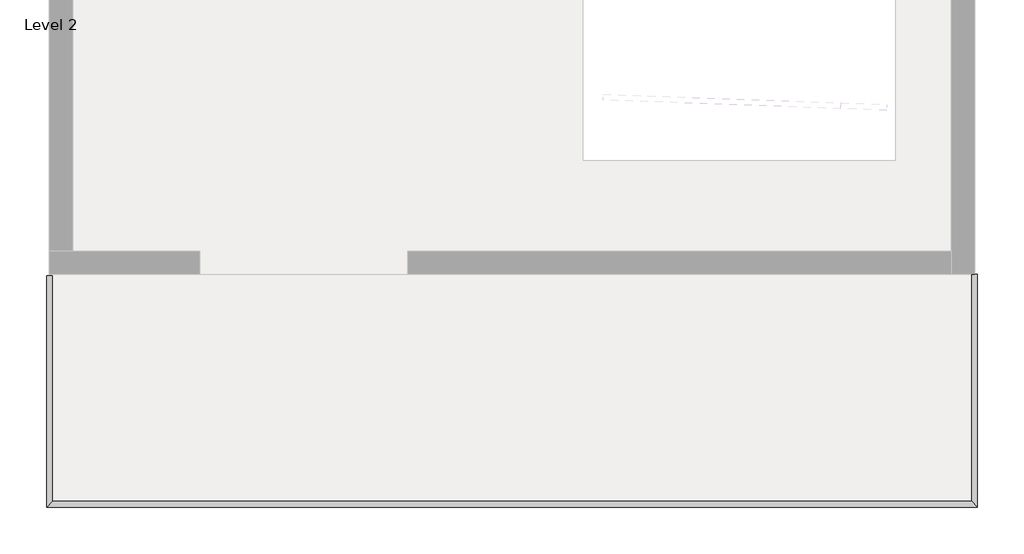
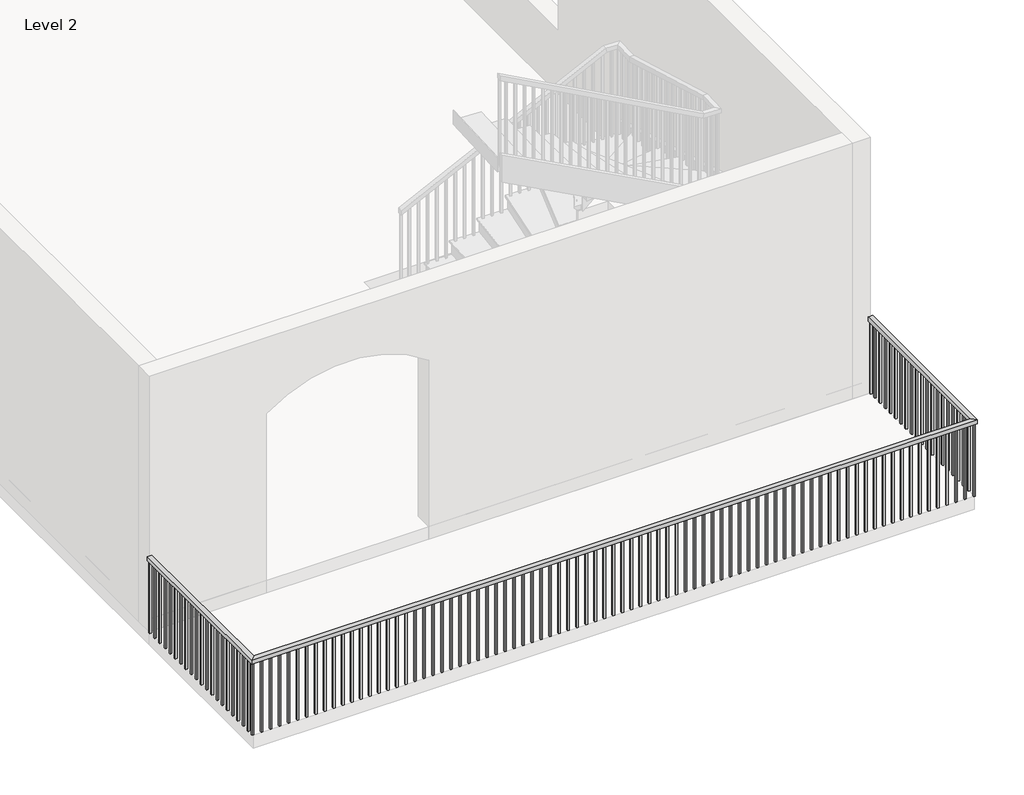
# One storey, part 2 of 3: 1 railing.
"""IFC4 building model written with IfcOpenShell, lengths in millimetres."""

from ifc_helpers import new_model, si_unit, frame, origin, place, context, project, spatial, polyline, outline, extrude, faceted_brep, element, save

model = new_model("IFC4")

# Units and contexts
model_context = context("Model", 3, world=origin())
ifc_project = project(units=[si_unit("LENGTHUNIT", "METRE", prefix="MILLI")], contexts=[model_context])

# Site, building, storey
site = spatial("IfcSite", under=ifc_project)
building = spatial("IfcBuilding", under=site)
storey = spatial("IfcBuildingStorey", under=building, Name="Level 2", Elevation=3048.0)

# Railing
placement = place(None, origin())
element("IfcRailing", 1, ObjectType="Handrail - Rectangular", at=placement, inside=storey, context=model_context, shape_type="SolidModel", body=[
    faceted_brep([(-14924.1126504, -4064.508, 3962.4), (-14924.1126504, -4064.508, 3911.6), (-14974.9126504, -4064.508, 3911.6), (-14974.9126504, -4064.508, 3962.4), (-14924.1126504, -6045.708, 3962.4), (-14924.1126504, -6045.708, 3911.6), (-14974.9126504, -6096.508, 3911.6), (-14974.9126504, -6096.508, 3962.4), (-6846.9126504, -6045.708, 3962.4), (-6846.9126504, -6045.708, 3911.6), (-6796.1126504, -6096.508, 3911.6), (-6796.1126504, -6096.508, 3962.4), (-6846.9126504, -4050.471143, 3962.4), (-6796.1126504, -4050.471143, 3962.4), (-6796.1126504, -4050.471143, 3911.6), (-6846.9126504, -4050.471143, 3911.6)], [[[0, 1, 2, 3]], [[1, 0, 4, 5]], [[2, 1, 5, 6]], [[3, 2, 6, 7]], [[0, 3, 7, 4]], [[5, 4, 8, 9]], [[6, 5, 9, 10]], [[7, 6, 10, 11]], [[4, 7, 11, 8]], [[12, 13, 14, 15]], [[9, 8, 12, 15]], [[10, 9, 15, 14]], [[11, 10, 14, 13]], [[8, 11, 13, 12]]]),
    extrude(outline(polyline([(-6811.9876504, -4150.233), (-6831.0376504, -4150.233), (-6831.0376504, -4131.183), (-6811.9876504, -4131.183), (-6811.9876504, -4150.233)])), frame((0.0, 0.0, 3048.0), z_axis=(0.0, 0.0, 1.0), x_axis=(1.0, 0.0, 0.0)), (0.0, 0.0, 1.0), 863.6),
    extrude(outline(polyline([(-6811.9876504, -4251.833), (-6831.0376504, -4251.833), (-6831.0376504, -4232.783), (-6811.9876504, -4232.783), (-6811.9876504, -4251.833)])), frame((0.0, 0.0, 3048.0), z_axis=(0.0, 0.0, 1.0), x_axis=(1.0, 0.0, 0.0)), (0.0, 0.0, 1.0), 863.6),
    extrude(outline(polyline([(-6811.9876504, -4353.433), (-6831.0376504, -4353.433), (-6831.0376504, -4334.383), (-6811.9876504, -4334.383), (-6811.9876504, -4353.433)])), frame((0.0, 0.0, 3048.0), z_axis=(0.0, 0.0, 1.0), x_axis=(1.0, 0.0, 0.0)), (0.0, 0.0, 1.0), 863.6),
    extrude(outline(polyline([(-6811.9876504, -4455.033), (-6831.0376504, -4455.033), (-6831.0376504, -4435.983), (-6811.9876504, -4435.983), (-6811.9876504, -4455.033)])), frame((0.0, 0.0, 3048.0), z_axis=(0.0, 0.0, 1.0), x_axis=(1.0, 0.0, 0.0)), (0.0, 0.0, 1.0), 863.6),
    extrude(outline(polyline([(-6811.9876504, -4556.633), (-6831.0376504, -4556.633), (-6831.0376504, -4537.583), (-6811.9876504, -4537.583), (-6811.9876504, -4556.633)])), frame((0.0, 0.0, 3048.0), z_axis=(0.0, 0.0, 1.0), x_axis=(1.0, 0.0, 0.0)), (0.0, 0.0, 1.0), 863.6),
    extrude(outline(polyline([(-6811.9876504, -4658.233), (-6831.0376504, -4658.233), (-6831.0376504, -4639.183), (-6811.9876504, -4639.183), (-6811.9876504, -4658.233)])), frame((0.0, 0.0, 3048.0), z_axis=(0.0, 0.0, 1.0), x_axis=(1.0, 0.0, 0.0)), (0.0, 0.0, 1.0), 863.6),
    extrude(outline(polyline([(-6811.9876504, -4759.833), (-6831.0376504, -4759.833), (-6831.0376504, -4740.783), (-6811.9876504, -4740.783), (-6811.9876504, -4759.833)])), frame((0.0, 0.0, 3048.0), z_axis=(0.0, 0.0, 1.0), x_axis=(1.0, 0.0, 0.0)), (0.0, 0.0, 1.0), 863.6),
    extrude(outline(polyline([(-6811.9876504, -4861.433), (-6831.0376504, -4861.433), (-6831.0376504, -4842.383), (-6811.9876504, -4842.383), (-6811.9876504, -4861.433)])), frame((0.0, 0.0, 3048.0), z_axis=(0.0, 0.0, 1.0), x_axis=(1.0, 0.0, 0.0)), (0.0, 0.0, 1.0), 863.6),
    extrude(outline(polyline([(-6811.9876504, -4963.033), (-6831.0376504, -4963.033), (-6831.0376504, -4943.983), (-6811.9876504, -4943.983), (-6811.9876504, -4963.033)])), frame((0.0, 0.0, 3048.0), z_axis=(0.0, 0.0, 1.0), x_axis=(1.0, 0.0, 0.0)), (0.0, 0.0, 1.0), 863.6),
    extrude(outline(polyline([(-6811.9876504, -5064.633), (-6831.0376504, -5064.633), (-6831.0376504, -5045.583), (-6811.9876504, -5045.583), (-6811.9876504, -5064.633)])), frame((0.0, 0.0, 3048.0), z_axis=(0.0, 0.0, 1.0), x_axis=(1.0, 0.0, 0.0)), (0.0, 0.0, 1.0), 863.6),
    extrude(outline(polyline([(-6811.9876504, -5166.233), (-6831.0376504, -5166.233), (-6831.0376504, -5147.183), (-6811.9876504, -5147.183), (-6811.9876504, -5166.233)])), frame((0.0, 0.0, 3048.0), z_axis=(0.0, 0.0, 1.0), x_axis=(1.0, 0.0, 0.0)), (0.0, 0.0, 1.0), 863.6),
    extrude(outline(polyline([(-6811.9876504, -5267.833), (-6831.0376504, -5267.833), (-6831.0376504, -5248.783), (-6811.9876504, -5248.783), (-6811.9876504, -5267.833)])), frame((0.0, 0.0, 3048.0), z_axis=(0.0, 0.0, 1.0), x_axis=(1.0, 0.0, 0.0)), (0.0, 0.0, 1.0), 863.6),
    extrude(outline(polyline([(-6811.9876504, -5369.433), (-6831.0376504, -5369.433), (-6831.0376504, -5350.383), (-6811.9876504, -5350.383), (-6811.9876504, -5369.433)])), frame((0.0, 0.0, 3048.0), z_axis=(0.0, 0.0, 1.0), x_axis=(1.0, 0.0, 0.0)), (0.0, 0.0, 1.0), 863.6),
    extrude(outline(polyline([(-6811.9876504, -5471.033), (-6831.0376504, -5471.033), (-6831.0376504, -5451.983), (-6811.9876504, -5451.983), (-6811.9876504, -5471.033)])), frame((0.0, 0.0, 3048.0), z_axis=(0.0, 0.0, 1.0), x_axis=(1.0, 0.0, 0.0)), (0.0, 0.0, 1.0), 863.6),
    extrude(outline(polyline([(-6811.9876504, -5572.633), (-6831.0376504, -5572.633), (-6831.0376504, -5553.583), (-6811.9876504, -5553.583), (-6811.9876504, -5572.633)])), frame((0.0, 0.0, 3048.0), z_axis=(0.0, 0.0, 1.0), x_axis=(1.0, 0.0, 0.0)), (0.0, 0.0, 1.0), 863.6),
    extrude(outline(polyline([(-6811.9876504, -5674.233), (-6831.0376504, -5674.233), (-6831.0376504, -5655.183), (-6811.9876504, -5655.183), (-6811.9876504, -5674.233)])), frame((0.0, 0.0, 3048.0), z_axis=(0.0, 0.0, 1.0), x_axis=(1.0, 0.0, 0.0)), (0.0, 0.0, 1.0), 863.6),
    extrude(outline(polyline([(-6811.9876504, -5775.833), (-6831.0376504, -5775.833), (-6831.0376504, -5756.783), (-6811.9876504, -5756.783), (-6811.9876504, -5775.833)])), frame((0.0, 0.0, 3048.0), z_axis=(0.0, 0.0, 1.0), x_axis=(1.0, 0.0, 0.0)), (0.0, 0.0, 1.0), 863.6),
    extrude(outline(polyline([(-6811.9876504, -5877.433), (-6831.0376504, -5877.433), (-6831.0376504, -5858.383), (-6811.9876504, -5858.383), (-6811.9876504, -5877.433)])), frame((0.0, 0.0, 3048.0), z_axis=(0.0, 0.0, 1.0), x_axis=(1.0, 0.0, 0.0)), (0.0, 0.0, 1.0), 863.6),
    extrude(outline(polyline([(-6811.9876504, -5979.033), (-6831.0376504, -5979.033), (-6831.0376504, -5959.983), (-6811.9876504, -5959.983), (-6811.9876504, -5979.033)])), frame((0.0, 0.0, 3048.0), z_axis=(0.0, 0.0, 1.0), x_axis=(1.0, 0.0, 0.0)), (0.0, 0.0, 1.0), 863.6),
    extrude(outline(polyline([(-6932.6376504, -6080.633), (-6932.6376504, -6061.583), (-6913.5876504, -6061.583), (-6913.5876504, -6080.633), (-6932.6376504, -6080.633)])), frame((0.0, 0.0, 3048.0), z_axis=(0.0, 0.0, 1.0), x_axis=(1.0, 0.0, 0.0)), (0.0, 0.0, 1.0), 863.6),
    extrude(outline(polyline([(-7034.2376504, -6080.633), (-7034.2376504, -6061.583), (-7015.1876504, -6061.583), (-7015.1876504, -6080.633), (-7034.2376504, -6080.633)])), frame((0.0, 0.0, 3048.0), z_axis=(0.0, 0.0, 1.0), x_axis=(1.0, 0.0, 0.0)), (0.0, 0.0, 1.0), 863.6),
    extrude(outline(polyline([(-7135.8376504, -6080.633), (-7135.8376504, -6061.583), (-7116.7876504, -6061.583), (-7116.7876504, -6080.633), (-7135.8376504, -6080.633)])), frame((0.0, 0.0, 3048.0), z_axis=(0.0, 0.0, 1.0), x_axis=(1.0, 0.0, 0.0)), (0.0, 0.0, 1.0), 863.6),
    extrude(outline(polyline([(-7237.4376504, -6080.633), (-7237.4376504, -6061.583), (-7218.3876504, -6061.583), (-7218.3876504, -6080.633), (-7237.4376504, -6080.633)])), frame((0.0, 0.0, 3048.0), z_axis=(0.0, 0.0, 1.0), x_axis=(1.0, 0.0, 0.0)), (0.0, 0.0, 1.0), 863.6),
    extrude(outline(polyline([(-7339.0376504, -6080.633), (-7339.0376504, -6061.583), (-7319.9876504, -6061.583), (-7319.9876504, -6080.633), (-7339.0376504, -6080.633)])), frame((0.0, 0.0, 3048.0), z_axis=(0.0, 0.0, 1.0), x_axis=(1.0, 0.0, 0.0)), (0.0, 0.0, 1.0), 863.6),
    extrude(outline(polyline([(-7440.6376504, -6080.633), (-7440.6376504, -6061.583), (-7421.5876504, -6061.583), (-7421.5876504, -6080.633), (-7440.6376504, -6080.633)])), frame((0.0, 0.0, 3048.0), z_axis=(0.0, 0.0, 1.0), x_axis=(1.0, 0.0, 0.0)), (0.0, 0.0, 1.0), 863.6),
    extrude(outline(polyline([(-7542.2376504, -6080.633), (-7542.2376504, -6061.583), (-7523.1876504, -6061.583), (-7523.1876504, -6080.633), (-7542.2376504, -6080.633)])), frame((0.0, 0.0, 3048.0), z_axis=(0.0, 0.0, 1.0), x_axis=(1.0, 0.0, 0.0)), (0.0, 0.0, 1.0), 863.6),
    extrude(outline(polyline([(-7643.8376504, -6080.633), (-7643.8376504, -6061.583), (-7624.7876504, -6061.583), (-7624.7876504, -6080.633), (-7643.8376504, -6080.633)])), frame((0.0, 0.0, 3048.0), z_axis=(0.0, 0.0, 1.0), x_axis=(1.0, 0.0, 0.0)), (0.0, 0.0, 1.0), 863.6),
    extrude(outline(polyline([(-7745.4376504, -6080.633), (-7745.4376504, -6061.583), (-7726.3876504, -6061.583), (-7726.3876504, -6080.633), (-7745.4376504, -6080.633)])), frame((0.0, 0.0, 3048.0), z_axis=(0.0, 0.0, 1.0), x_axis=(1.0, 0.0, 0.0)), (0.0, 0.0, 1.0), 863.6),
    extrude(outline(polyline([(-7847.0376504, -6080.633), (-7847.0376504, -6061.583), (-7827.9876504, -6061.583), (-7827.9876504, -6080.633), (-7847.0376504, -6080.633)])), frame((0.0, 0.0, 3048.0), z_axis=(0.0, 0.0, 1.0), x_axis=(1.0, 0.0, 0.0)), (0.0, 0.0, 1.0), 863.6),
    extrude(outline(polyline([(-7948.6376504, -6080.633), (-7948.6376504, -6061.583), (-7929.5876504, -6061.583), (-7929.5876504, -6080.633), (-7948.6376504, -6080.633)])), frame((0.0, 0.0, 3048.0), z_axis=(0.0, 0.0, 1.0), x_axis=(1.0, 0.0, 0.0)), (0.0, 0.0, 1.0), 863.6),
    extrude(outline(polyline([(-8050.2376504, -6080.633), (-8050.2376504, -6061.583), (-8031.1876504, -6061.583), (-8031.1876504, -6080.633), (-8050.2376504, -6080.633)])), frame((0.0, 0.0, 3048.0), z_axis=(0.0, 0.0, 1.0), x_axis=(1.0, 0.0, 0.0)), (0.0, 0.0, 1.0), 863.6),
    extrude(outline(polyline([(-8151.8376504, -6080.633), (-8151.8376504, -6061.583), (-8132.7876504, -6061.583), (-8132.7876504, -6080.633), (-8151.8376504, -6080.633)])), frame((0.0, 0.0, 3048.0), z_axis=(0.0, 0.0, 1.0), x_axis=(1.0, 0.0, 0.0)), (0.0, 0.0, 1.0), 863.6),
    extrude(outline(polyline([(-8253.4376504, -6080.633), (-8253.4376504, -6061.583), (-8234.3876504, -6061.583), (-8234.3876504, -6080.633), (-8253.4376504, -6080.633)])), frame((0.0, 0.0, 3048.0), z_axis=(0.0, 0.0, 1.0), x_axis=(1.0, 0.0, 0.0)), (0.0, 0.0, 1.0), 863.6),
    extrude(outline(polyline([(-8355.0376504, -6080.633), (-8355.0376504, -6061.583), (-8335.9876504, -6061.583), (-8335.9876504, -6080.633), (-8355.0376504, -6080.633)])), frame((0.0, 0.0, 3048.0), z_axis=(0.0, 0.0, 1.0), x_axis=(1.0, 0.0, 0.0)), (0.0, 0.0, 1.0), 863.6),
    extrude(outline(polyline([(-8456.6376504, -6080.633), (-8456.6376504, -6061.583), (-8437.5876504, -6061.583), (-8437.5876504, -6080.633), (-8456.6376504, -6080.633)])), frame((0.0, 0.0, 3048.0), z_axis=(0.0, 0.0, 1.0), x_axis=(1.0, 0.0, 0.0)), (0.0, 0.0, 1.0), 863.6),
    extrude(outline(polyline([(-8558.2376504, -6080.633), (-8558.2376504, -6061.583), (-8539.1876504, -6061.583), (-8539.1876504, -6080.633), (-8558.2376504, -6080.633)])), frame((0.0, 0.0, 3048.0), z_axis=(0.0, 0.0, 1.0), x_axis=(1.0, 0.0, 0.0)), (0.0, 0.0, 1.0), 863.6),
    extrude(outline(polyline([(-8659.8376504, -6080.633), (-8659.8376504, -6061.583), (-8640.7876504, -6061.583), (-8640.7876504, -6080.633), (-8659.8376504, -6080.633)])), frame((0.0, 0.0, 3048.0), z_axis=(0.0, 0.0, 1.0), x_axis=(1.0, 0.0, 0.0)), (0.0, 0.0, 1.0), 863.6),
    extrude(outline(polyline([(-8761.4376504, -6080.633), (-8761.4376504, -6061.583), (-8742.3876504, -6061.583), (-8742.3876504, -6080.633), (-8761.4376504, -6080.633)])), frame((0.0, 0.0, 3048.0), z_axis=(0.0, 0.0, 1.0), x_axis=(1.0, 0.0, 0.0)), (0.0, 0.0, 1.0), 863.6),
    extrude(outline(polyline([(-8863.0376504, -6080.633), (-8863.0376504, -6061.583), (-8843.9876504, -6061.583), (-8843.9876504, -6080.633), (-8863.0376504, -6080.633)])), frame((0.0, 0.0, 3048.0), z_axis=(0.0, 0.0, 1.0), x_axis=(1.0, 0.0, 0.0)), (0.0, 0.0, 1.0), 863.6),
    extrude(outline(polyline([(-8964.6376504, -6080.633), (-8964.6376504, -6061.583), (-8945.5876504, -6061.583), (-8945.5876504, -6080.633), (-8964.6376504, -6080.633)])), frame((0.0, 0.0, 3048.0), z_axis=(0.0, 0.0, 1.0), x_axis=(1.0, 0.0, 0.0)), (0.0, 0.0, 1.0), 863.6),
    extrude(outline(polyline([(-9066.2376504, -6080.633), (-9066.2376504, -6061.583), (-9047.1876504, -6061.583), (-9047.1876504, -6080.633), (-9066.2376504, -6080.633)])), frame((0.0, 0.0, 3048.0), z_axis=(0.0, 0.0, 1.0), x_axis=(1.0, 0.0, 0.0)), (0.0, 0.0, 1.0), 863.6),
    extrude(outline(polyline([(-9167.8376504, -6080.633), (-9167.8376504, -6061.583), (-9148.7876504, -6061.583), (-9148.7876504, -6080.633), (-9167.8376504, -6080.633)])), frame((0.0, 0.0, 3048.0), z_axis=(0.0, 0.0, 1.0), x_axis=(1.0, 0.0, 0.0)), (0.0, 0.0, 1.0), 863.6),
    extrude(outline(polyline([(-9269.4376504, -6080.633), (-9269.4376504, -6061.583), (-9250.3876504, -6061.583), (-9250.3876504, -6080.633), (-9269.4376504, -6080.633)])), frame((0.0, 0.0, 3048.0), z_axis=(0.0, 0.0, 1.0), x_axis=(1.0, 0.0, 0.0)), (0.0, 0.0, 1.0), 863.6),
    extrude(outline(polyline([(-9371.0376504, -6080.633), (-9371.0376504, -6061.583), (-9351.9876504, -6061.583), (-9351.9876504, -6080.633), (-9371.0376504, -6080.633)])), frame((0.0, 0.0, 3048.0), z_axis=(0.0, 0.0, 1.0), x_axis=(1.0, 0.0, 0.0)), (0.0, 0.0, 1.0), 863.6),
    extrude(outline(polyline([(-9472.6376504, -6080.633), (-9472.6376504, -6061.583), (-9453.5876504, -6061.583), (-9453.5876504, -6080.633), (-9472.6376504, -6080.633)])), frame((0.0, 0.0, 3048.0), z_axis=(0.0, 0.0, 1.0), x_axis=(1.0, 0.0, 0.0)), (0.0, 0.0, 1.0), 863.6),
    extrude(outline(polyline([(-9574.2376504, -6080.633), (-9574.2376504, -6061.583), (-9555.1876504, -6061.583), (-9555.1876504, -6080.633), (-9574.2376504, -6080.633)])), frame((0.0, 0.0, 3048.0), z_axis=(0.0, 0.0, 1.0), x_axis=(1.0, 0.0, 0.0)), (0.0, 0.0, 1.0), 863.6),
    extrude(outline(polyline([(-9675.8376504, -6080.633), (-9675.8376504, -6061.583), (-9656.7876504, -6061.583), (-9656.7876504, -6080.633), (-9675.8376504, -6080.633)])), frame((0.0, 0.0, 3048.0), z_axis=(0.0, 0.0, 1.0), x_axis=(1.0, 0.0, 0.0)), (0.0, 0.0, 1.0), 863.6),
    extrude(outline(polyline([(-9777.4376504, -6080.633), (-9777.4376504, -6061.583), (-9758.3876504, -6061.583), (-9758.3876504, -6080.633), (-9777.4376504, -6080.633)])), frame((0.0, 0.0, 3048.0), z_axis=(0.0, 0.0, 1.0), x_axis=(1.0, 0.0, 0.0)), (0.0, 0.0, 1.0), 863.6),
    extrude(outline(polyline([(-9879.0376504, -6080.633), (-9879.0376504, -6061.583), (-9859.9876504, -6061.583), (-9859.9876504, -6080.633), (-9879.0376504, -6080.633)])), frame((0.0, 0.0, 3048.0), z_axis=(0.0, 0.0, 1.0), x_axis=(1.0, 0.0, 0.0)), (0.0, 0.0, 1.0), 863.6),
    extrude(outline(polyline([(-9980.6376504, -6080.633), (-9980.6376504, -6061.583), (-9961.5876504, -6061.583), (-9961.5876504, -6080.633), (-9980.6376504, -6080.633)])), frame((0.0, 0.0, 3048.0), z_axis=(0.0, 0.0, 1.0), x_axis=(1.0, 0.0, 0.0)), (0.0, 0.0, 1.0), 863.6),
    extrude(outline(polyline([(-10082.2376504, -6080.633), (-10082.2376504, -6061.583), (-10063.1876504, -6061.583), (-10063.1876504, -6080.633), (-10082.2376504, -6080.633)])), frame((0.0, 0.0, 3048.0), z_axis=(0.0, 0.0, 1.0), x_axis=(1.0, 0.0, 0.0)), (0.0, 0.0, 1.0), 863.6),
    extrude(outline(polyline([(-10183.8376504, -6080.633), (-10183.8376504, -6061.583), (-10164.7876504, -6061.583), (-10164.7876504, -6080.633), (-10183.8376504, -6080.633)])), frame((0.0, 0.0, 3048.0), z_axis=(0.0, 0.0, 1.0), x_axis=(1.0, 0.0, 0.0)), (0.0, 0.0, 1.0), 863.6),
    extrude(outline(polyline([(-10285.4376504, -6080.633), (-10285.4376504, -6061.583), (-10266.3876504, -6061.583), (-10266.3876504, -6080.633), (-10285.4376504, -6080.633)])), frame((0.0, 0.0, 3048.0), z_axis=(0.0, 0.0, 1.0), x_axis=(1.0, 0.0, 0.0)), (0.0, 0.0, 1.0), 863.6),
    extrude(outline(polyline([(-10387.0376504, -6080.633), (-10387.0376504, -6061.583), (-10367.9876504, -6061.583), (-10367.9876504, -6080.633), (-10387.0376504, -6080.633)])), frame((0.0, 0.0, 3048.0), z_axis=(0.0, 0.0, 1.0), x_axis=(1.0, 0.0, 0.0)), (0.0, 0.0, 1.0), 863.6),
    extrude(outline(polyline([(-10488.6376504, -6080.633), (-10488.6376504, -6061.583), (-10469.5876504, -6061.583), (-10469.5876504, -6080.633), (-10488.6376504, -6080.633)])), frame((0.0, 0.0, 3048.0), z_axis=(0.0, 0.0, 1.0), x_axis=(1.0, 0.0, 0.0)), (0.0, 0.0, 1.0), 863.6),
    extrude(outline(polyline([(-10590.2376504, -6080.633), (-10590.2376504, -6061.583), (-10571.1876504, -6061.583), (-10571.1876504, -6080.633), (-10590.2376504, -6080.633)])), frame((0.0, 0.0, 3048.0), z_axis=(0.0, 0.0, 1.0), x_axis=(1.0, 0.0, 0.0)), (0.0, 0.0, 1.0), 863.6),
    extrude(outline(polyline([(-10691.8376504, -6080.633), (-10691.8376504, -6061.583), (-10672.7876504, -6061.583), (-10672.7876504, -6080.633), (-10691.8376504, -6080.633)])), frame((0.0, 0.0, 3048.0), z_axis=(0.0, 0.0, 1.0), x_axis=(1.0, 0.0, 0.0)), (0.0, 0.0, 1.0), 863.6),
    extrude(outline(polyline([(-10793.4376504, -6080.633), (-10793.4376504, -6061.583), (-10774.3876504, -6061.583), (-10774.3876504, -6080.633), (-10793.4376504, -6080.633)])), frame((0.0, 0.0, 3048.0), z_axis=(0.0, 0.0, 1.0), x_axis=(1.0, 0.0, 0.0)), (0.0, 0.0, 1.0), 863.6),
    extrude(outline(polyline([(-10895.0376504, -6080.633), (-10895.0376504, -6061.583), (-10875.9876504, -6061.583), (-10875.9876504, -6080.633), (-10895.0376504, -6080.633)])), frame((0.0, 0.0, 3048.0), z_axis=(0.0, 0.0, 1.0), x_axis=(1.0, 0.0, 0.0)), (0.0, 0.0, 1.0), 863.6),
    extrude(outline(polyline([(-10996.6376504, -6080.633), (-10996.6376504, -6061.583), (-10977.5876504, -6061.583), (-10977.5876504, -6080.633), (-10996.6376504, -6080.633)])), frame((0.0, 0.0, 3048.0), z_axis=(0.0, 0.0, 1.0), x_axis=(1.0, 0.0, 0.0)), (0.0, 0.0, 1.0), 863.6),
    extrude(outline(polyline([(-11098.2376504, -6080.633), (-11098.2376504, -6061.583), (-11079.1876504, -6061.583), (-11079.1876504, -6080.633), (-11098.2376504, -6080.633)])), frame((0.0, 0.0, 3048.0), z_axis=(0.0, 0.0, 1.0), x_axis=(1.0, 0.0, 0.0)), (0.0, 0.0, 1.0), 863.6),
    extrude(outline(polyline([(-11199.8376504, -6080.633), (-11199.8376504, -6061.583), (-11180.7876504, -6061.583), (-11180.7876504, -6080.633), (-11199.8376504, -6080.633)])), frame((0.0, 0.0, 3048.0), z_axis=(0.0, 0.0, 1.0), x_axis=(1.0, 0.0, 0.0)), (0.0, 0.0, 1.0), 863.6),
    extrude(outline(polyline([(-11301.4376504, -6080.633), (-11301.4376504, -6061.583), (-11282.3876504, -6061.583), (-11282.3876504, -6080.633), (-11301.4376504, -6080.633)])), frame((0.0, 0.0, 3048.0), z_axis=(0.0, 0.0, 1.0), x_axis=(1.0, 0.0, 0.0)), (0.0, 0.0, 1.0), 863.6),
    extrude(outline(polyline([(-11403.0376504, -6080.633), (-11403.0376504, -6061.583), (-11383.9876504, -6061.583), (-11383.9876504, -6080.633), (-11403.0376504, -6080.633)])), frame((0.0, 0.0, 3048.0), z_axis=(0.0, 0.0, 1.0), x_axis=(1.0, 0.0, 0.0)), (0.0, 0.0, 1.0), 863.6),
    extrude(outline(polyline([(-11504.6376504, -6080.633), (-11504.6376504, -6061.583), (-11485.5876504, -6061.583), (-11485.5876504, -6080.633), (-11504.6376504, -6080.633)])), frame((0.0, 0.0, 3048.0), z_axis=(0.0, 0.0, 1.0), x_axis=(1.0, 0.0, 0.0)), (0.0, 0.0, 1.0), 863.6),
    extrude(outline(polyline([(-11606.2376504, -6080.633), (-11606.2376504, -6061.583), (-11587.1876504, -6061.583), (-11587.1876504, -6080.633), (-11606.2376504, -6080.633)])), frame((0.0, 0.0, 3048.0), z_axis=(0.0, 0.0, 1.0), x_axis=(1.0, 0.0, 0.0)), (0.0, 0.0, 1.0), 863.6),
    extrude(outline(polyline([(-11707.8376504, -6080.633), (-11707.8376504, -6061.583), (-11688.7876504, -6061.583), (-11688.7876504, -6080.633), (-11707.8376504, -6080.633)])), frame((0.0, 0.0, 3048.0), z_axis=(0.0, 0.0, 1.0), x_axis=(1.0, 0.0, 0.0)), (0.0, 0.0, 1.0), 863.6),
    extrude(outline(polyline([(-11809.4376504, -6080.633), (-11809.4376504, -6061.583), (-11790.3876504, -6061.583), (-11790.3876504, -6080.633), (-11809.4376504, -6080.633)])), frame((0.0, 0.0, 3048.0), z_axis=(0.0, 0.0, 1.0), x_axis=(1.0, 0.0, 0.0)), (0.0, 0.0, 1.0), 863.6),
    extrude(outline(polyline([(-11911.0376504, -6080.633), (-11911.0376504, -6061.583), (-11891.9876504, -6061.583), (-11891.9876504, -6080.633), (-11911.0376504, -6080.633)])), frame((0.0, 0.0, 3048.0), z_axis=(0.0, 0.0, 1.0), x_axis=(1.0, 0.0, 0.0)), (0.0, 0.0, 1.0), 863.6),
    extrude(outline(polyline([(-12012.6376504, -6080.633), (-12012.6376504, -6061.583), (-11993.5876504, -6061.583), (-11993.5876504, -6080.633), (-12012.6376504, -6080.633)])), frame((0.0, 0.0, 3048.0), z_axis=(0.0, 0.0, 1.0), x_axis=(1.0, 0.0, 0.0)), (0.0, 0.0, 1.0), 863.6),
    extrude(outline(polyline([(-12114.2376504, -6080.633), (-12114.2376504, -6061.583), (-12095.1876504, -6061.583), (-12095.1876504, -6080.633), (-12114.2376504, -6080.633)])), frame((0.0, 0.0, 3048.0), z_axis=(0.0, 0.0, 1.0), x_axis=(1.0, 0.0, 0.0)), (0.0, 0.0, 1.0), 863.6),
    extrude(outline(polyline([(-12215.8376504, -6080.633), (-12215.8376504, -6061.583), (-12196.7876504, -6061.583), (-12196.7876504, -6080.633), (-12215.8376504, -6080.633)])), frame((0.0, 0.0, 3048.0), z_axis=(0.0, 0.0, 1.0), x_axis=(1.0, 0.0, 0.0)), (0.0, 0.0, 1.0), 863.6),
    extrude(outline(polyline([(-12317.4376504, -6080.633), (-12317.4376504, -6061.583), (-12298.3876504, -6061.583), (-12298.3876504, -6080.633), (-12317.4376504, -6080.633)])), frame((0.0, 0.0, 3048.0), z_axis=(0.0, 0.0, 1.0), x_axis=(1.0, 0.0, 0.0)), (0.0, 0.0, 1.0), 863.6),
    extrude(outline(polyline([(-12419.0376504, -6080.633), (-12419.0376504, -6061.583), (-12399.9876504, -6061.583), (-12399.9876504, -6080.633), (-12419.0376504, -6080.633)])), frame((0.0, 0.0, 3048.0), z_axis=(0.0, 0.0, 1.0), x_axis=(1.0, 0.0, 0.0)), (0.0, 0.0, 1.0), 863.6),
    extrude(outline(polyline([(-12520.6376504, -6080.633), (-12520.6376504, -6061.583), (-12501.5876504, -6061.583), (-12501.5876504, -6080.633), (-12520.6376504, -6080.633)])), frame((0.0, 0.0, 3048.0), z_axis=(0.0, 0.0, 1.0), x_axis=(1.0, 0.0, 0.0)), (0.0, 0.0, 1.0), 863.6),
    extrude(outline(polyline([(-12622.2376504, -6080.633), (-12622.2376504, -6061.583), (-12603.1876504, -6061.583), (-12603.1876504, -6080.633), (-12622.2376504, -6080.633)])), frame((0.0, 0.0, 3048.0), z_axis=(0.0, 0.0, 1.0), x_axis=(1.0, 0.0, 0.0)), (0.0, 0.0, 1.0), 863.6),
    extrude(outline(polyline([(-12723.8376504, -6080.633), (-12723.8376504, -6061.583), (-12704.7876504, -6061.583), (-12704.7876504, -6080.633), (-12723.8376504, -6080.633)])), frame((0.0, 0.0, 3048.0), z_axis=(0.0, 0.0, 1.0), x_axis=(1.0, 0.0, 0.0)), (0.0, 0.0, 1.0), 863.6),
    extrude(outline(polyline([(-12825.4376504, -6080.633), (-12825.4376504, -6061.583), (-12806.3876504, -6061.583), (-12806.3876504, -6080.633), (-12825.4376504, -6080.633)])), frame((0.0, 0.0, 3048.0), z_axis=(0.0, 0.0, 1.0), x_axis=(1.0, 0.0, 0.0)), (0.0, 0.0, 1.0), 863.6),
    extrude(outline(polyline([(-12927.0376504, -6080.633), (-12927.0376504, -6061.583), (-12907.9876504, -6061.583), (-12907.9876504, -6080.633), (-12927.0376504, -6080.633)])), frame((0.0, 0.0, 3048.0), z_axis=(0.0, 0.0, 1.0), x_axis=(1.0, 0.0, 0.0)), (0.0, 0.0, 1.0), 863.6),
    extrude(outline(polyline([(-13028.6376504, -6080.633), (-13028.6376504, -6061.583), (-13009.5876504, -6061.583), (-13009.5876504, -6080.633), (-13028.6376504, -6080.633)])), frame((0.0, 0.0, 3048.0), z_axis=(0.0, 0.0, 1.0), x_axis=(1.0, 0.0, 0.0)), (0.0, 0.0, 1.0), 863.6),
    extrude(outline(polyline([(-13130.2376504, -6080.633), (-13130.2376504, -6061.583), (-13111.1876504, -6061.583), (-13111.1876504, -6080.633), (-13130.2376504, -6080.633)])), frame((0.0, 0.0, 3048.0), z_axis=(0.0, 0.0, 1.0), x_axis=(1.0, 0.0, 0.0)), (0.0, 0.0, 1.0), 863.6),
    extrude(outline(polyline([(-13231.8376504, -6080.633), (-13231.8376504, -6061.583), (-13212.7876504, -6061.583), (-13212.7876504, -6080.633), (-13231.8376504, -6080.633)])), frame((0.0, 0.0, 3048.0), z_axis=(0.0, 0.0, 1.0), x_axis=(1.0, 0.0, 0.0)), (0.0, 0.0, 1.0), 863.6),
    extrude(outline(polyline([(-13333.4376504, -6080.633), (-13333.4376504, -6061.583), (-13314.3876504, -6061.583), (-13314.3876504, -6080.633), (-13333.4376504, -6080.633)])), frame((0.0, 0.0, 3048.0), z_axis=(0.0, 0.0, 1.0), x_axis=(1.0, 0.0, 0.0)), (0.0, 0.0, 1.0), 863.6),
    extrude(outline(polyline([(-13435.0376504, -6080.633), (-13435.0376504, -6061.583), (-13415.9876504, -6061.583), (-13415.9876504, -6080.633), (-13435.0376504, -6080.633)])), frame((0.0, 0.0, 3048.0), z_axis=(0.0, 0.0, 1.0), x_axis=(1.0, 0.0, 0.0)), (0.0, 0.0, 1.0), 863.6),
    extrude(outline(polyline([(-13536.6376504, -6080.633), (-13536.6376504, -6061.583), (-13517.5876504, -6061.583), (-13517.5876504, -6080.633), (-13536.6376504, -6080.633)])), frame((0.0, 0.0, 3048.0), z_axis=(0.0, 0.0, 1.0), x_axis=(1.0, 0.0, 0.0)), (0.0, 0.0, 1.0), 863.6),
    extrude(outline(polyline([(-13638.2376504, -6080.633), (-13638.2376504, -6061.583), (-13619.1876504, -6061.583), (-13619.1876504, -6080.633), (-13638.2376504, -6080.633)])), frame((0.0, 0.0, 3048.0), z_axis=(0.0, 0.0, 1.0), x_axis=(1.0, 0.0, 0.0)), (0.0, 0.0, 1.0), 863.6),
    extrude(outline(polyline([(-13739.8376504, -6080.633), (-13739.8376504, -6061.583), (-13720.7876504, -6061.583), (-13720.7876504, -6080.633), (-13739.8376504, -6080.633)])), frame((0.0, 0.0, 3048.0), z_axis=(0.0, 0.0, 1.0), x_axis=(1.0, 0.0, 0.0)), (0.0, 0.0, 1.0), 863.6),
    extrude(outline(polyline([(-13841.4376504, -6080.633), (-13841.4376504, -6061.583), (-13822.3876504, -6061.583), (-13822.3876504, -6080.633), (-13841.4376504, -6080.633)])), frame((0.0, 0.0, 3048.0), z_axis=(0.0, 0.0, 1.0), x_axis=(1.0, 0.0, 0.0)), (0.0, 0.0, 1.0), 863.6),
    extrude(outline(polyline([(-13943.0376504, -6080.633), (-13943.0376504, -6061.583), (-13923.9876504, -6061.583), (-13923.9876504, -6080.633), (-13943.0376504, -6080.633)])), frame((0.0, 0.0, 3048.0), z_axis=(0.0, 0.0, 1.0), x_axis=(1.0, 0.0, 0.0)), (0.0, 0.0, 1.0), 863.6),
    extrude(outline(polyline([(-14044.6376504, -6080.633), (-14044.6376504, -6061.583), (-14025.5876504, -6061.583), (-14025.5876504, -6080.633), (-14044.6376504, -6080.633)])), frame((0.0, 0.0, 3048.0), z_axis=(0.0, 0.0, 1.0), x_axis=(1.0, 0.0, 0.0)), (0.0, 0.0, 1.0), 863.6),
    extrude(outline(polyline([(-14146.2376504, -6080.633), (-14146.2376504, -6061.583), (-14127.1876504, -6061.583), (-14127.1876504, -6080.633), (-14146.2376504, -6080.633)])), frame((0.0, 0.0, 3048.0), z_axis=(0.0, 0.0, 1.0), x_axis=(1.0, 0.0, 0.0)), (0.0, 0.0, 1.0), 863.6),
    extrude(outline(polyline([(-14247.8376504, -6080.633), (-14247.8376504, -6061.583), (-14228.7876504, -6061.583), (-14228.7876504, -6080.633), (-14247.8376504, -6080.633)])), frame((0.0, 0.0, 3048.0), z_axis=(0.0, 0.0, 1.0), x_axis=(1.0, 0.0, 0.0)), (0.0, 0.0, 1.0), 863.6),
    extrude(outline(polyline([(-14349.4376504, -6080.633), (-14349.4376504, -6061.583), (-14330.3876504, -6061.583), (-14330.3876504, -6080.633), (-14349.4376504, -6080.633)])), frame((0.0, 0.0, 3048.0), z_axis=(0.0, 0.0, 1.0), x_axis=(1.0, 0.0, 0.0)), (0.0, 0.0, 1.0), 863.6),
    extrude(outline(polyline([(-14451.0376504, -6080.633), (-14451.0376504, -6061.583), (-14431.9876504, -6061.583), (-14431.9876504, -6080.633), (-14451.0376504, -6080.633)])), frame((0.0, 0.0, 3048.0), z_axis=(0.0, 0.0, 1.0), x_axis=(1.0, 0.0, 0.0)), (0.0, 0.0, 1.0), 863.6),
    extrude(outline(polyline([(-14552.6376504, -6080.633), (-14552.6376504, -6061.583), (-14533.5876504, -6061.583), (-14533.5876504, -6080.633), (-14552.6376504, -6080.633)])), frame((0.0, 0.0, 3048.0), z_axis=(0.0, 0.0, 1.0), x_axis=(1.0, 0.0, 0.0)), (0.0, 0.0, 1.0), 863.6),
    extrude(outline(polyline([(-14654.2376504, -6080.633), (-14654.2376504, -6061.583), (-14635.1876504, -6061.583), (-14635.1876504, -6080.633), (-14654.2376504, -6080.633)])), frame((0.0, 0.0, 3048.0), z_axis=(0.0, 0.0, 1.0), x_axis=(1.0, 0.0, 0.0)), (0.0, 0.0, 1.0), 863.6),
    extrude(outline(polyline([(-14755.8376504, -6080.633), (-14755.8376504, -6061.583), (-14736.7876504, -6061.583), (-14736.7876504, -6080.633), (-14755.8376504, -6080.633)])), frame((0.0, 0.0, 3048.0), z_axis=(0.0, 0.0, 1.0), x_axis=(1.0, 0.0, 0.0)), (0.0, 0.0, 1.0), 863.6),
    extrude(outline(polyline([(-14857.4376504, -6080.633), (-14857.4376504, -6061.583), (-14838.3876504, -6061.583), (-14838.3876504, -6080.633), (-14857.4376504, -6080.633)])), frame((0.0, 0.0, 3048.0), z_axis=(0.0, 0.0, 1.0), x_axis=(1.0, 0.0, 0.0)), (0.0, 0.0, 1.0), 863.6),
    extrude(outline(polyline([(-14959.0376504, -5985.383), (-14939.9876504, -5985.383), (-14939.9876504, -6004.433), (-14959.0376504, -6004.433), (-14959.0376504, -5985.383)])), frame((0.0, 0.0, 3048.0), z_axis=(0.0, 0.0, 1.0), x_axis=(1.0, 0.0, 0.0)), (0.0, 0.0, 1.0), 863.6),
    extrude(outline(polyline([(-14959.0376504, -5883.783), (-14939.9876504, -5883.783), (-14939.9876504, -5902.833), (-14959.0376504, -5902.833), (-14959.0376504, -5883.783)])), frame((0.0, 0.0, 3048.0), z_axis=(0.0, 0.0, 1.0), x_axis=(1.0, 0.0, 0.0)), (0.0, 0.0, 1.0), 863.6),
    extrude(outline(polyline([(-14959.0376504, -5782.183), (-14939.9876504, -5782.183), (-14939.9876504, -5801.233), (-14959.0376504, -5801.233), (-14959.0376504, -5782.183)])), frame((0.0, 0.0, 3048.0), z_axis=(0.0, 0.0, 1.0), x_axis=(1.0, 0.0, 0.0)), (0.0, 0.0, 1.0), 863.6),
    extrude(outline(polyline([(-14959.0376504, -5680.583), (-14939.9876504, -5680.583), (-14939.9876504, -5699.633), (-14959.0376504, -5699.633), (-14959.0376504, -5680.583)])), frame((0.0, 0.0, 3048.0), z_axis=(0.0, 0.0, 1.0), x_axis=(1.0, 0.0, 0.0)), (0.0, 0.0, 1.0), 863.6),
    extrude(outline(polyline([(-14959.0376504, -5578.983), (-14939.9876504, -5578.983), (-14939.9876504, -5598.033), (-14959.0376504, -5598.033), (-14959.0376504, -5578.983)])), frame((0.0, 0.0, 3048.0), z_axis=(0.0, 0.0, 1.0), x_axis=(1.0, 0.0, 0.0)), (0.0, 0.0, 1.0), 863.6),
    extrude(outline(polyline([(-14959.0376504, -5477.383), (-14939.9876504, -5477.383), (-14939.9876504, -5496.433), (-14959.0376504, -5496.433), (-14959.0376504, -5477.383)])), frame((0.0, 0.0, 3048.0), z_axis=(0.0, 0.0, 1.0), x_axis=(1.0, 0.0, 0.0)), (0.0, 0.0, 1.0), 863.6),
    extrude(outline(polyline([(-14959.0376504, -5375.783), (-14939.9876504, -5375.783), (-14939.9876504, -5394.833), (-14959.0376504, -5394.833), (-14959.0376504, -5375.783)])), frame((0.0, 0.0, 3048.0), z_axis=(0.0, 0.0, 1.0), x_axis=(1.0, 0.0, 0.0)), (0.0, 0.0, 1.0), 863.6),
    extrude(outline(polyline([(-14959.0376504, -5274.183), (-14939.9876504, -5274.183), (-14939.9876504, -5293.233), (-14959.0376504, -5293.233), (-14959.0376504, -5274.183)])), frame((0.0, 0.0, 3048.0), z_axis=(0.0, 0.0, 1.0), x_axis=(1.0, 0.0, 0.0)), (0.0, 0.0, 1.0), 863.6),
    extrude(outline(polyline([(-14959.0376504, -5172.583), (-14939.9876504, -5172.583), (-14939.9876504, -5191.633), (-14959.0376504, -5191.633), (-14959.0376504, -5172.583)])), frame((0.0, 0.0, 3048.0), z_axis=(0.0, 0.0, 1.0), x_axis=(1.0, 0.0, 0.0)), (0.0, 0.0, 1.0), 863.6),
    extrude(outline(polyline([(-14959.0376504, -5070.983), (-14939.9876504, -5070.983), (-14939.9876504, -5090.033), (-14959.0376504, -5090.033), (-14959.0376504, -5070.983)])), frame((0.0, 0.0, 3048.0), z_axis=(0.0, 0.0, 1.0), x_axis=(1.0, 0.0, 0.0)), (0.0, 0.0, 1.0), 863.6),
    extrude(outline(polyline([(-14959.0376504, -4969.383), (-14939.9876504, -4969.383), (-14939.9876504, -4988.433), (-14959.0376504, -4988.433), (-14959.0376504, -4969.383)])), frame((0.0, 0.0, 3048.0), z_axis=(0.0, 0.0, 1.0), x_axis=(1.0, 0.0, 0.0)), (0.0, 0.0, 1.0), 863.6),
    extrude(outline(polyline([(-14959.0376504, -4867.783), (-14939.9876504, -4867.783), (-14939.9876504, -4886.833), (-14959.0376504, -4886.833), (-14959.0376504, -4867.783)])), frame((0.0, 0.0, 3048.0), z_axis=(0.0, 0.0, 1.0), x_axis=(1.0, 0.0, 0.0)), (0.0, 0.0, 1.0), 863.6),
    extrude(outline(polyline([(-14959.0376504, -4766.183), (-14939.9876504, -4766.183), (-14939.9876504, -4785.233), (-14959.0376504, -4785.233), (-14959.0376504, -4766.183)])), frame((0.0, 0.0, 3048.0), z_axis=(0.0, 0.0, 1.0), x_axis=(1.0, 0.0, 0.0)), (0.0, 0.0, 1.0), 863.6),
    extrude(outline(polyline([(-14959.0376504, -4664.583), (-14939.9876504, -4664.583), (-14939.9876504, -4683.633), (-14959.0376504, -4683.633), (-14959.0376504, -4664.583)])), frame((0.0, 0.0, 3048.0), z_axis=(0.0, 0.0, 1.0), x_axis=(1.0, 0.0, 0.0)), (0.0, 0.0, 1.0), 863.6),
    extrude(outline(polyline([(-14959.0376504, -4562.983), (-14939.9876504, -4562.983), (-14939.9876504, -4582.033), (-14959.0376504, -4582.033), (-14959.0376504, -4562.983)])), frame((0.0, 0.0, 3048.0), z_axis=(0.0, 0.0, 1.0), x_axis=(1.0, 0.0, 0.0)), (0.0, 0.0, 1.0), 863.6),
    extrude(outline(polyline([(-14959.0376504, -4461.383), (-14939.9876504, -4461.383), (-14939.9876504, -4480.433), (-14959.0376504, -4480.433), (-14959.0376504, -4461.383)])), frame((0.0, 0.0, 3048.0), z_axis=(0.0, 0.0, 1.0), x_axis=(1.0, 0.0, 0.0)), (0.0, 0.0, 1.0), 863.6),
    extrude(outline(polyline([(-14959.0376504, -4359.783), (-14939.9876504, -4359.783), (-14939.9876504, -4378.833), (-14959.0376504, -4378.833), (-14959.0376504, -4359.783)])), frame((0.0, 0.0, 3048.0), z_axis=(0.0, 0.0, 1.0), x_axis=(1.0, 0.0, 0.0)), (0.0, 0.0, 1.0), 863.6),
    extrude(outline(polyline([(-14959.0376504, -4258.183), (-14939.9876504, -4258.183), (-14939.9876504, -4277.233), (-14959.0376504, -4277.233), (-14959.0376504, -4258.183)])), frame((0.0, 0.0, 3048.0), z_axis=(0.0, 0.0, 1.0), x_axis=(1.0, 0.0, 0.0)), (0.0, 0.0, 1.0), 863.6),
    extrude(outline(polyline([(-14959.0376504, -4156.583), (-14939.9876504, -4156.583), (-14939.9876504, -4175.633), (-14959.0376504, -4175.633), (-14959.0376504, -4156.583)])), frame((0.0, 0.0, 3048.0), z_axis=(0.0, 0.0, 1.0), x_axis=(1.0, 0.0, 0.0)), (0.0, 0.0, 1.0), 863.6),
    extrude(outline(polyline([(-6831.0376504, -6080.633), (-6831.0376504, -6061.583), (-6811.9876504, -6061.583), (-6811.9876504, -6080.633), (-6831.0376504, -6080.633)])), frame((0.0, 0.0, 3048.0), z_axis=(0.0, 0.0, 1.0), x_axis=(1.0, 0.0, 0.0)), (0.0, 0.0, 1.0), 863.6),
    extrude(outline(polyline([(-14959.0376504, -6061.583), (-14939.9876504, -6061.583), (-14939.9876504, -6080.633), (-14959.0376504, -6080.633), (-14959.0376504, -6061.583)])), frame((0.0, 0.0, 3048.0), z_axis=(0.0, 0.0, 1.0), x_axis=(1.0, 0.0, 0.0)), (0.0, 0.0, 1.0), 863.6),
    extrude(outline(polyline([(-6811.9876504, -4069.521143), (-6831.0376504, -4069.521143), (-6831.0376504, -4050.471143), (-6811.9876504, -4050.471143), (-6811.9876504, -4069.521143)])), frame((0.0, 0.0, 3048.0), z_axis=(0.0, 0.0, 1.0), x_axis=(1.0, 0.0, 0.0)), (0.0, 0.0, 1.0), 863.6),
    extrude(outline(polyline([(-14959.0376504, -4064.508), (-14939.9876504, -4064.508), (-14939.9876504, -4083.558), (-14959.0376504, -4083.558), (-14959.0376504, -4064.508)])), frame((0.0, 0.0, 3048.0), z_axis=(0.0, 0.0, 1.0), x_axis=(1.0, 0.0, 0.0)), (0.0, 0.0, 1.0), 863.6),
])

save(model, "model.ifc")

# Revit data of these elements
# Type "Handrail - Rectangular"
#   Assembly Code = "C2010400"
#   built-in parameter 1008612 = 0.0416667 (stored number, unit not read)
#   built-in parameter 1008611 = 0.0416667 (stored number, unit not read)
#   built-in parameter 1008609 = 0.333333 (stored number, unit not read)
#   built-in parameter 1008604 = 0.166667 (stored number, unit not read)
#   built-in parameter 1008603 = 0.166667 (stored number, unit not read)
#   Railing Height = 3' - 0"
#   built-in parameter 1008630 = 2
#   built-in parameter 1008610 = 2
#   built-in parameter 1008618 = Baluster - Square : 3/4"
# Element 1 (IfcRailing, "Handrail - Rectangular")
#   Phase Created = New Construction
